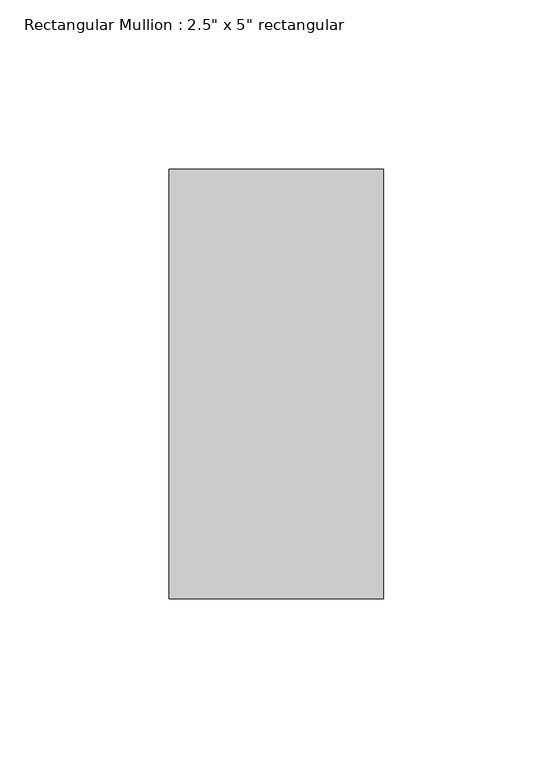
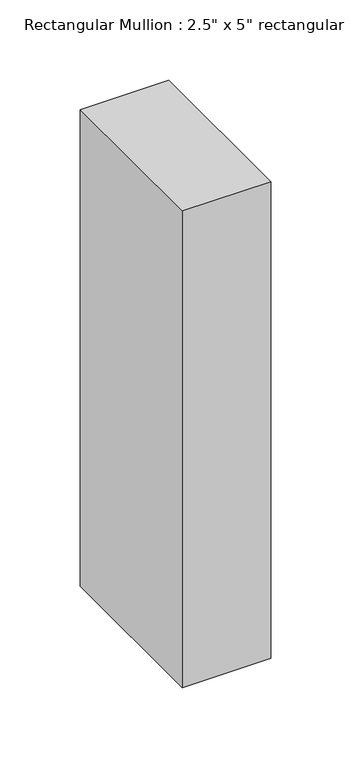
"""IFC4 building model written with IfcOpenShell, lengths in millimetres: member geometry."""

from ifc_helpers import new_model, si_unit, frame, origin, place, context, project, spatial, polyline, outline, extrude, source, transform, mapped, element, save


def member_0417a2a7(model_context):
    return source(origin(), model_context, "Body", "SweptSolid", [
        extrude(outline(polyline([(0.0, 63.5), (0.0, -63.5), (-63.5, -63.5), (-63.5, 63.5), (0.0, 63.5)])), frame((0.0, 0.0, -362.6039559), z_axis=(0.0, 0.0, 1.0), x_axis=(1.0, 0.0, 0.0)), (0.0, 0.0, 1.0), 362.6039559),
    ])


if __name__ == "__main__":
    model = new_model("IFC4")
    model_context = context("Model", 3, world=origin())
    ifc_project = project(units=[si_unit("LENGTHUNIT", "METRE", prefix="MILLI")], contexts=[model_context])
    site = spatial("IfcSite", under=ifc_project)
    building = spatial("IfcBuilding", under=site)
    placement = place(None, origin())
    member_shape = member_0417a2a7(model_context)
    element("IfcMember", 1, ObjectType="Rectangular Mullion : 2.5\" x 5\" rectangular", at=placement, inside=building, context=model_context, shape_type="MappedRepresentation", body=[
        mapped(member_shape, transform((0.0, 0.0, 0.0), x_axis=(1.0, 0.0, 0.0), y_axis=(0.0, 1.0, 0.0), z_axis=(0.0, 0.0, 1.0))),
    ])
    save(model, "model.ifc")

# Revit data of these elements
# Type "Rectangular Mullion : 2.5\" x 5\" rectangular"
#   built-in parameter 1007304 = 0.416667 (stored number, unit not read)
#   built-in parameter 1007301 = 0.104167 (stored number, unit not read)
#   built-in parameter 1007300 = 0.104167 (stored number, unit not read)
# Element 1 (IfcMember, "Rectangular Mullion : 2.5\" x 5\" rectangular")
#   Materials on its faces: "Aluminum"
# Materials
#   "Aluminum": class "Metal", colour RGB 247 247 247, transparency 0, Description = "Aluminum 6061", Cost = 0
